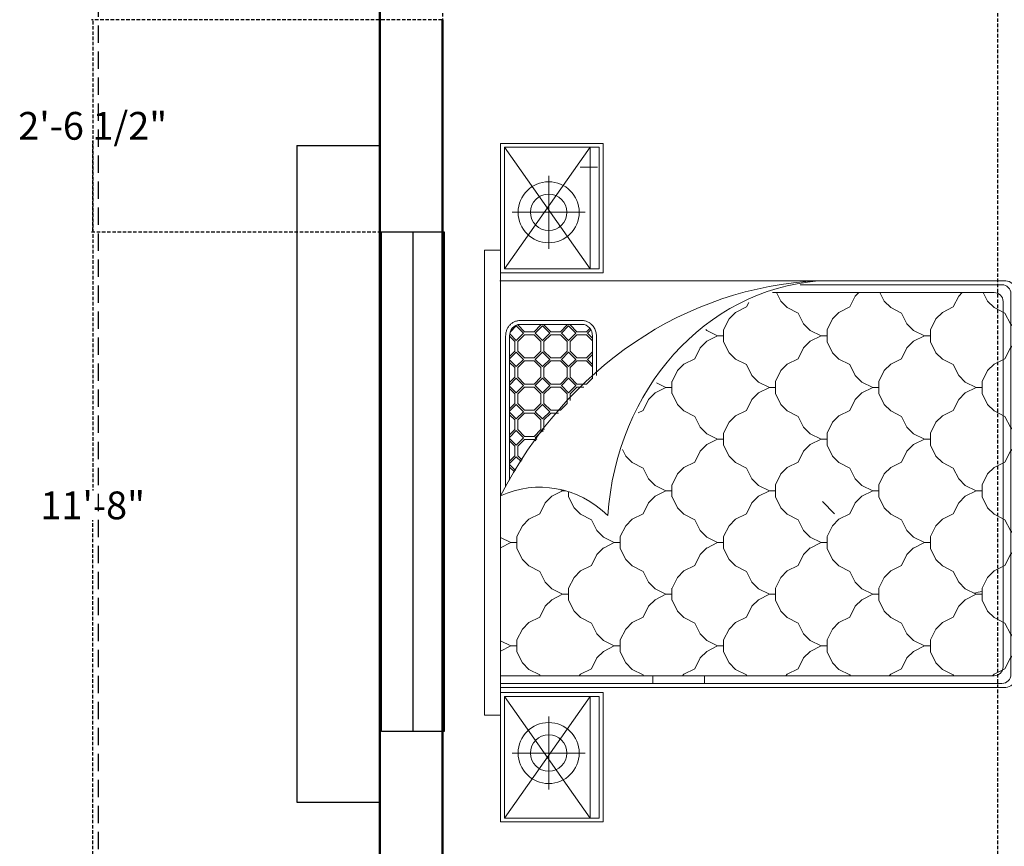
# Model space of a CAD drawing. Units: inches. Extents: x 513 to 1142, y 396 to 927.
# Tile 2 of 31: x 523 to 665, y 518 to 637. Entities that reach past the tile are written whole.
import ezdxf

# ---------------------------------------------------------------- set-up
doc = ezdxf.new("R2010")
doc.units = ezdxf.units.IN
doc.header["$MEASUREMENT"] = 0
doc.linetypes.add('DASHED', pattern=[0.75, 0.5, -0.25])
for name, color, linetype, lineweight in [('A-ANNO-DIMS', 2, 'DASHED', 18), ('A-WALL', 7, 'Continuous', 50), ('furniture', 92, 'Continuous', 18), ('windows', 172, 'Continuous', 25)]:
    doc.layers.add(name, color=color, linetype=linetype, lineweight=lineweight)
doc.styles.get("Standard").update_dxf_attribs({"font": 'arial.ttf'})
doc.dimstyles.get("Standard").update_dxf_attribs({"dimtxt": 4, "dimasz": 0.18, "dimexe": 0.18, "dimexo": 0.0625, "dimgap": 0.09, "dimtad": 0, "dimtih": 1, "dimtoh": 1, "dimdec": 0, "dimrnd": 6, "dimzin": 0, "dimdsep": 46, "dimlunit": 3, "dimtxsty": 'Standard', "dimcen": 0.09, "dimadec": 0, "dimazin": 0, "dimtfac": 1, "dimtdec": 0, "dimtofl": 0, "dimtmove": 0, "dimatfit": 3, "dimfxl": 1, "dimtolj": 1, "dimtzin": 0, "dimarcsym": 0})

# ---------------------------------------------------------------- blocks, each defined once
blk = doc.blocks.new('A$C029D5C69')
for p, q in [((0.4164, 2.0693), (0.4164, 2.0066)), ((2.2315, 2.0693), (0.4164, 2.0693)), ((2.2315, 2.0066), (2.2315, 2.0693)), ((0, 1.606), (0, 2.0066)), ((0, 2.0066), (0.505, 2.0066)), ((0.4164, 2.0066), (2.2315, 2.0066)), ((0.505, 2.0066), (0.505, 1.606)), ((0.5252, 0.0351), (0.5252, 2.0066)), ((0.5403, 0.0502), (0.5403, 2.0066)), ((0.5706, 0.0805), (0.5706, 2.0066)), ((0.6869, 1.966), (0.6666, 2.0066)), ((0.7072, 2.0066), (0.6869, 1.966)), ((1.0902, 1.966), (1.0699, 2.0066)), ((1.1106, 2.0066), (1.0902, 1.966)), ((2.1114, 2.0087), (2.1114, 0.0351)), ((2.6479, 2.0066), (2.1429, 2.0066)), ((2.1429, 2.0066), (2.1429, 1.606)), ((2.6479, 1.606), (2.6479, 2.0066)), ((0.0151, 1.6211), (0.0151, 1.9915)), ((0.0151, 1.9915), (0.4899, 1.9915)), ((0.2689, 1.9609), (0.2689, 1.6764)), ((0.4899, 1.9915), (0.4899, 1.6211)), ((0.6869, 1.9425), (0.6869, 1.966)), ((0.6869, 1.9425), (0.6869, 1.966)), ((1.0902, 1.9425), (1.0902, 1.966)), ((1.0902, 1.9425), (1.0902, 1.966)), ((1.8954, 1.9865), (1.3081, 1.9865)), ((1.8954, 1.9713), (1.3339, 1.9713)), ((1.3849, 1.9713), (1.3656, 1.952)), ((1.3945, 1.9713), (1.3714, 1.9483)), ((1.4249, 1.945), (1.3986, 1.9713)), ((1.4288, 1.9507), (1.4081, 1.9713)), ((1.487, 1.9713), (1.4664, 1.9507)), ((1.4966, 1.9713), (1.4703, 1.945)), ((1.527, 1.945), (1.5007, 1.9713)), ((1.5309, 1.9507), (1.5102, 1.9713)), ((1.5891, 1.9713), (1.5685, 1.9507)), ((1.5987, 1.9713), (1.5724, 1.945)), ((1.6291, 1.945), (1.6028, 1.9713)), ((1.633, 1.9507), (1.6123, 1.9713)), ((1.6912, 1.9713), (1.6706, 1.9507)), ((1.7008, 1.9713), (1.6745, 1.945)), ((1.7312, 1.945), (1.7049, 1.9713)), ((1.7351, 1.9507), (1.7144, 1.9713)), ((1.7933, 1.9713), (1.7727, 1.9507)), ((1.8029, 1.9713), (1.7766, 1.945)), ((1.8333, 1.945), (1.807, 1.9713)), ((1.8372, 1.9507), (1.8165, 1.9713)), ((1.8954, 1.9713), (1.8748, 1.9507)), ((1.9043, 1.9707), (1.8787, 1.945)), ((1.9354, 1.945), (1.9114, 1.969)), ((2.6328, 1.9915), (2.158, 1.9915)), ((2.158, 1.9915), (2.158, 1.6211)), ((2.379, 1.9609), (2.379, 1.6764)), ((2.6328, 1.6211), (2.6328, 1.9915)), ((0.621, 1.9213), (0.5955, 1.8958)), ((0.6634, 1.9425), (0.621, 1.9213)), ((0.6634, 1.9425), (0.621, 1.9213)), ((0.6869, 1.9425), (0.6634, 1.9425)), ((0.6869, 1.9425), (0.7104, 1.9425)), ((0.7528, 1.9213), (0.7104, 1.9425)), ((0.7528, 1.9213), (0.7104, 1.9425)), ((0.7783, 1.8958), (0.7528, 1.9213)), ((1.0243, 1.9213), (0.9988, 1.8958)), ((1.0668, 1.9425), (1.0244, 1.9213)), ((1.0668, 1.9425), (1.0244, 1.9213)), ((1.0902, 1.9425), (1.0668, 1.9425)), ((1.0902, 1.9425), (1.1137, 1.9425)), ((1.1561, 1.9213), (1.1137, 1.9425)), ((1.1561, 1.9213), (1.1137, 1.9425)), ((1.1816, 1.8958), (1.1561, 1.9213)), ((1.4249, 1.945), (1.4059, 1.926)), ((1.4288, 1.9394), (1.4116, 1.9222)), ((1.4476, 1.9507), (1.4288, 1.9507)), ((1.4288, 1.9393), (1.4476, 1.9393)), ((1.4476, 1.9507), (1.4664, 1.9507)), ((1.4664, 1.9393), (1.4476, 1.9393)), ((1.493, 1.9128), (1.4664, 1.9394)), ((1.4986, 1.9167), (1.4703, 1.945)), ((1.527, 1.945), (1.4986, 1.9167)), ((1.5309, 1.9394), (1.5043, 1.9128)), ((1.5497, 1.9507), (1.5309, 1.9507)), ((1.5309, 1.9393), (1.5497, 1.9393)), ((1.5497, 1.9507), (1.5685, 1.9507)), ((1.5685, 1.9393), (1.5497, 1.9393)), ((1.595, 1.9128), (1.5685, 1.9394)), ((1.6007, 1.9167), (1.5724, 1.945)), ((1.6291, 1.945), (1.6007, 1.9167)), ((1.633, 1.9394), (1.6064, 1.9128)), ((1.6518, 1.9507), (1.633, 1.9507)), ((1.633, 1.9393), (1.6518, 1.9393)), ((1.6518, 1.9507), (1.6706, 1.9507)), ((1.6706, 1.9393), (1.6518, 1.9393)), ((1.6971, 1.9128), (1.6706, 1.9394)), ((1.7028, 1.9167), (1.6745, 1.945)), ((1.7312, 1.945), (1.7028, 1.9167)), ((1.7351, 1.9394), (1.7085, 1.9128)), ((1.7539, 1.9507), (1.7351, 1.9507)), ((1.7351, 1.9393), (1.7539, 1.9393)), ((1.7539, 1.9507), (1.7727, 1.9507)), ((1.7727, 1.9393), (1.7539, 1.9393)), ((1.7992, 1.9128), (1.7727, 1.9394)), ((1.8049, 1.9167), (1.7766, 1.945)), ((1.8333, 1.945), (1.8049, 1.9167)), ((1.8372, 1.9394), (1.8106, 1.9128)), ((1.856, 1.9507), (1.8372, 1.9507)), ((1.8372, 1.9393), (1.856, 1.9393)), ((1.856, 1.9507), (1.8748, 1.9507)), ((1.8748, 1.9393), (1.856, 1.9393)), ((1.9013, 1.9128), (1.8748, 1.9394)), ((1.907, 1.9167), (1.8787, 1.945)), ((1.9354, 1.945), (1.907, 1.9167)), ((1.9393, 1.9394), (1.9127, 1.9128)), ((1.9393, 1.9393), (1.9404, 1.9393)), ((1.9414, 1.688), (1.9414, 1.931)), ((1.9565, 1.688), (1.9565, 1.931)), ((0.5955, 1.8958), (0.5743, 1.8534)), ((0.7995, 1.8534), (0.7783, 1.8958)), ((0.9989, 1.8958), (0.9777, 1.8534)), ((1.2028, 1.8534), (1.1816, 1.8958)), ((1.493, 1.8752), (1.493, 1.9128)), ((1.5043, 1.8752), (1.5043, 1.9128)), ((1.595, 1.8752), (1.595, 1.9128)), ((1.6064, 1.8752), (1.6064, 1.9128)), ((1.6971, 1.8752), (1.6971, 1.9128)), ((1.7085, 1.8752), (1.7085, 1.9128)), ((1.7992, 1.8752), (1.7992, 1.9128)), ((1.8106, 1.8752), (1.8106, 1.9128)), ((1.9013, 1.8752), (1.9013, 1.9128)), ((1.9127, 1.8752), (1.9127, 1.9128)), ((0.5743, 1.8534), (0.5706, 1.8515)), ((0.5743, 1.8534), (0.5706, 1.8515)), ((0.8419, 1.8322), (0.7995, 1.8534)), ((0.8419, 1.8322), (0.7995, 1.8534)), ((0.9777, 1.8534), (0.9353, 1.8322)), ((0.9777, 1.8534), (0.9353, 1.8322)), ((1.2452, 1.8322), (1.2028, 1.8534)), ((1.2452, 1.8322), (1.2028, 1.8534)), ((1.493, 1.8752), (1.4867, 1.869)), ((1.4986, 1.8713), (1.4922, 1.8648)), ((1.527, 1.8429), (1.4986, 1.8713)), ((1.5309, 1.8486), (1.5043, 1.8752)), ((1.5497, 1.8486), (1.5309, 1.8486)), ((1.5497, 1.8486), (1.5685, 1.8486)), ((1.595, 1.8752), (1.5685, 1.8486)), ((1.6007, 1.8713), (1.5724, 1.8429)), ((1.6291, 1.8429), (1.6007, 1.8713)), ((1.633, 1.8486), (1.6064, 1.8752)), ((1.6518, 1.8486), (1.633, 1.8486)), ((1.6518, 1.8486), (1.6706, 1.8486)), ((1.6971, 1.8752), (1.6706, 1.8486)), ((1.7028, 1.8713), (1.6745, 1.8429)), ((1.7312, 1.8429), (1.7028, 1.8713)), ((1.7351, 1.8486), (1.7085, 1.8752)), ((1.7539, 1.8486), (1.7351, 1.8486)), ((1.7539, 1.8486), (1.7727, 1.8486)), ((1.7992, 1.8752), (1.7727, 1.8486)), ((1.8049, 1.8713), (1.7766, 1.8429)), ((1.8333, 1.8429), (1.8049, 1.8713)), ((1.8372, 1.8486), (1.8106, 1.8752)), ((1.856, 1.8486), (1.8372, 1.8486)), ((1.856, 1.8486), (1.8748, 1.8486)), ((1.9013, 1.8752), (1.8748, 1.8486)), ((1.907, 1.8713), (1.8787, 1.8429)), ((1.9354, 1.8429), (1.907, 1.8713)), ((1.9393, 1.8486), (1.9127, 1.8752)), ((1.9414, 1.8486), (1.9393, 1.8486)), ((0.1267, 1.8186), (0.4111, 1.8186)), ((0.8674, 1.8067), (0.8419, 1.8322)), ((0.8886, 1.7643), (0.8674, 1.8067)), ((0.9098, 1.8067), (0.8886, 1.7643)), ((0.9352, 1.8322), (0.9097, 1.8067)), ((1.2707, 1.8067), (1.2452, 1.8322)), ((1.2919, 1.7643), (1.2707, 1.8067)), ((1.527, 1.8429), (1.5242, 1.8401)), ((1.5309, 1.8373), (1.5295, 1.8359)), ((1.5309, 1.8373), (1.5497, 1.8373)), ((1.5685, 1.8373), (1.5497, 1.8373)), ((1.595, 1.8107), (1.5685, 1.8373)), ((1.6007, 1.8146), (1.5724, 1.8429)), ((1.595, 1.7806), (1.595, 1.8107)), ((1.6291, 1.8429), (1.6007, 1.8146)), ((1.633, 1.8373), (1.6064, 1.8107)), ((1.6064, 1.7731), (1.6064, 1.8107)), ((1.633, 1.8373), (1.6518, 1.8373)), ((1.6706, 1.8373), (1.6518, 1.8373)), ((1.6971, 1.8107), (1.6706, 1.8373)), ((1.7028, 1.8146), (1.6745, 1.8429)), ((1.6971, 1.7731), (1.6971, 1.8107)), ((1.7312, 1.8429), (1.7028, 1.8146)), ((1.7351, 1.8373), (1.7085, 1.8107)), ((1.7085, 1.7731), (1.7085, 1.8107)), ((1.7351, 1.8373), (1.7539, 1.8373)), ((1.7727, 1.8373), (1.7539, 1.8373)), ((1.7992, 1.8107), (1.7727, 1.8373)), ((1.8049, 1.8146), (1.7766, 1.8429)), ((1.7992, 1.7731), (1.7992, 1.8107)), ((1.8333, 1.8429), (1.8049, 1.8146)), ((1.8372, 1.8373), (1.8106, 1.8107)), ((1.8106, 1.7731), (1.8106, 1.8107)), ((1.8372, 1.8373), (1.856, 1.8373)), ((1.8748, 1.8373), (1.856, 1.8373)), ((1.9013, 1.8107), (1.8748, 1.8373)), ((1.907, 1.8146), (1.8787, 1.8429)), ((1.9013, 1.7731), (1.9013, 1.8107)), ((1.9354, 1.8429), (1.907, 1.8146)), ((1.9393, 1.8373), (1.9127, 1.8107)), ((1.9127, 1.7731), (1.9127, 1.8107)), ((1.9393, 1.8373), (1.9414, 1.8373)), ((2.2367, 1.8186), (2.5212, 1.8186)), ((1.2981, 1.7768), (1.2919, 1.7643)), ((1.633, 1.7465), (1.6064, 1.7731)), ((1.6971, 1.7731), (1.6706, 1.7465)), ((1.7028, 1.7692), (1.6745, 1.7408)), ((1.7312, 1.7408), (1.7028, 1.7692)), ((1.7351, 1.7465), (1.7085, 1.7731)), ((1.7992, 1.7731), (1.7727, 1.7465)), ((1.8049, 1.7692), (1.7766, 1.7408)), ((1.8333, 1.7408), (1.8049, 1.7692)), ((1.8372, 1.7465), (1.8106, 1.7731)), ((1.9013, 1.7731), (1.8748, 1.7465)), ((1.907, 1.7692), (1.8787, 1.7408)), ((1.9354, 1.7408), (1.907, 1.7692)), ((1.9393, 1.7465), (1.9127, 1.7731)), ((0.8651, 1.7408), (0.8227, 1.7196)), ((0.8651, 1.7408), (0.8227, 1.7196)), ((0.912, 1.7408), (0.8651, 1.7408)), ((0.8886, 1.7408), (0.8886, 1.7643)), ((0.9544, 1.7196), (0.912, 1.7408)), ((0.9544, 1.7196), (0.912, 1.7408)), ((1.2684, 1.7408), (1.226, 1.7196)), ((1.2684, 1.7408), (1.226, 1.7196)), ((1.2885, 1.7408), (1.2684, 1.7408)), ((1.2919, 1.7519), (1.2919, 1.7643)), ((1.6518, 1.7465), (1.633, 1.7465)), ((1.6443, 1.7352), (1.6518, 1.7352)), ((1.6518, 1.7465), (1.6706, 1.7465)), ((1.6706, 1.7352), (1.6518, 1.7352)), ((1.6971, 1.7086), (1.6706, 1.7352)), ((1.7028, 1.7125), (1.6745, 1.7408)), ((1.7312, 1.7408), (1.7028, 1.7125)), ((1.7351, 1.7352), (1.7085, 1.7086)), ((1.7539, 1.7465), (1.7351, 1.7465)), ((1.7351, 1.7352), (1.7539, 1.7352)), ((1.7539, 1.7465), (1.7727, 1.7465)), ((1.7727, 1.7352), (1.7539, 1.7352)), ((1.7992, 1.7086), (1.7727, 1.7352)), ((1.8049, 1.7125), (1.7766, 1.7408)), ((1.8333, 1.7408), (1.8049, 1.7125)), ((1.8372, 1.7352), (1.8106, 1.7086)), ((1.856, 1.7465), (1.8372, 1.7465)), ((1.8372, 1.7352), (1.856, 1.7352)), ((1.856, 1.7465), (1.8748, 1.7465)), ((1.8748, 1.7352), (1.856, 1.7352)), ((1.9013, 1.7086), (1.8748, 1.7352)), ((1.907, 1.7125), (1.8787, 1.7408)), ((1.9354, 1.7408), (1.907, 1.7125)), ((1.9393, 1.7352), (1.9127, 1.7086)), ((1.9414, 1.7465), (1.9393, 1.7465)), ((1.9393, 1.7352), (1.9414, 1.7352)), ((0.5766, 1.6941), (0.5706, 1.7002)), ((0.5978, 1.6517), (0.5766, 1.6941)), ((0.7972, 1.6941), (0.776, 1.6517)), ((0.8227, 1.7196), (0.7972, 1.6941)), ((0.98, 1.6941), (0.9545, 1.7196)), ((1.0011, 1.6517), (0.9799, 1.6941)), ((1.2005, 1.6941), (1.1793, 1.6517)), ((1.226, 1.7196), (1.2005, 1.6941)), ((1.6971, 1.682), (1.6971, 1.7086)), ((1.7085, 1.671), (1.7085, 1.7086)), ((1.7992, 1.671), (1.7992, 1.7086)), ((1.8106, 1.671), (1.8106, 1.7086)), ((1.9013, 1.671), (1.9013, 1.7086)), ((1.9127, 1.671), (1.9127, 1.7086)), ((2.5551, 1.6275), (2.5551, 1.696)), ((1.7318, 1.6477), (1.7085, 1.671)), ((1.7992, 1.671), (1.7759, 1.6477)), ((1.8049, 1.6671), (1.7855, 1.6477)), ((1.8244, 1.6477), (1.8049, 1.6671)), ((1.8339, 1.6477), (1.8106, 1.671)), ((1.9013, 1.671), (1.878, 1.6477)), ((1.907, 1.6671), (1.8876, 1.6477)), ((1.9202, 1.6539), (1.907, 1.6671)), ((1.926, 1.6577), (1.9127, 1.671)), ((0.4899, 1.6211), (0.0151, 1.6211)), ((0.6402, 1.6305), (0.5978, 1.6517)), ((0.6402, 1.6305), (0.5978, 1.6517)), ((0.6657, 1.605), (0.6402, 1.6305)), ((0.7336, 1.6305), (0.7081, 1.605)), ((0.776, 1.6517), (0.7336, 1.6305)), ((0.776, 1.6517), (0.7336, 1.6305)), ((1.0435, 1.6305), (1.0011, 1.6517)), ((1.0435, 1.6305), (1.0011, 1.6517)), ((1.0691, 1.605), (1.0436, 1.6305)), ((1.1369, 1.6305), (1.1114, 1.605)), ((1.1793, 1.6517), (1.1369, 1.6305)), ((1.1793, 1.6517), (1.1369, 1.6305)), ((1.8961, 1.6477), (1.7289, 1.6477)), ((1.8961, 1.6325), (1.7422, 1.6325)), ((2.158, 1.6211), (2.6328, 1.6211)), ((0.505, 1.606), (0, 1.606)), ((0.6869, 1.5626), (0.6657, 1.605)), ((0.7081, 1.605), (0.6869, 1.5626)), ((1.0902, 1.5626), (1.069, 1.605)), ((1.1114, 1.605), (1.0902, 1.5626)), ((2.1429, 1.606), (2.6479, 1.606)), ((0.6634, 1.5391), (0.621, 1.5179)), ((0.6634, 1.5391), (0.621, 1.5179)), ((0.6869, 1.5392), (0.6634, 1.5392)), ((0.6869, 1.5392), (0.6869, 1.5626)), ((0.6869, 1.5392), (0.6869, 1.5626)), ((0.6869, 1.5392), (0.7104, 1.5392)), ((0.7528, 1.5179), (0.7104, 1.5391)), ((0.7528, 1.5179), (0.7104, 1.5391)), ((1.0668, 1.5391), (1.0244, 1.5179)), ((1.0668, 1.5391), (1.0244, 1.5179)), ((1.0902, 1.5392), (1.0668, 1.5392)), ((1.0902, 1.5392), (1.0902, 1.5626)), ((1.0902, 1.5392), (1.0902, 1.5626)), ((1.0902, 1.5392), (1.1137, 1.5392)), ((1.1561, 1.5179), (1.1137, 1.5391)), ((1.1561, 1.5179), (1.1137, 1.5391)), ((0.621, 1.5179), (0.5955, 1.4924)), ((0.7783, 1.4924), (0.7528, 1.5179)), ((1.0243, 1.5179), (0.9988, 1.4924)), ((1.1816, 1.4924), (1.1561, 1.5179)), ((1.4277, 1.5179), (1.4022, 1.4924)), ((1.4534, 1.5308), (1.4277, 1.5179)), ((1.4534, 1.5308), (1.4277, 1.5179)), ((0.5955, 1.4925), (0.5743, 1.4501)), ((0.7995, 1.4501), (0.7783, 1.4925)), ((0.9989, 1.4925), (0.9777, 1.4501)), ((1.2028, 1.4501), (1.1816, 1.4925)), ((1.4022, 1.4925), (1.381, 1.4501)), ((1.6062, 1.4501), (1.5966, 1.4692)), ((0.5743, 1.45), (0.5706, 1.4481)), ((0.5743, 1.45), (0.5706, 1.4481)), ((0.8419, 1.4288), (0.7995, 1.45)), ((0.8419, 1.4288), (0.7995, 1.45)), ((0.8674, 1.4033), (0.8419, 1.4288)), ((0.9352, 1.4288), (0.9097, 1.4033)), ((0.9777, 1.45), (0.9353, 1.4288)), ((0.9777, 1.45), (0.9353, 1.4288)), ((1.2452, 1.4288), (1.2028, 1.45)), ((1.2452, 1.4288), (1.2028, 1.45)), ((1.2707, 1.4033), (1.2452, 1.4288)), ((1.3386, 1.4288), (1.3131, 1.4033)), ((1.381, 1.45), (1.3386, 1.4288)), ((1.381, 1.45), (1.3386, 1.4288)), ((1.6486, 1.4288), (1.6062, 1.45)), ((1.6486, 1.4288), (1.6062, 1.45)), ((1.6741, 1.4033), (1.6486, 1.4288)), ((0.5403, 1.4117), (0.5706, 1.4117)), ((0.8886, 1.361), (0.8674, 1.4034)), ((0.9098, 1.4034), (0.8886, 1.361)), ((1.2919, 1.361), (1.2707, 1.4034)), ((1.3131, 1.4034), (1.2919, 1.361)), ((1.6953, 1.361), (1.6741, 1.4034)), ((1.714, 1.3984), (1.6953, 1.361)), ((0.8886, 1.3375), (0.8886, 1.3609)), ((1.2919, 1.3375), (1.2919, 1.3609)), ((1.6953, 1.3375), (1.6953, 1.3609)), ((0.8227, 1.3163), (0.7972, 1.2908)), ((0.8651, 1.3374), (0.8227, 1.3162)), ((0.8651, 1.3374), (0.8227, 1.3162)), ((0.912, 1.3375), (0.8651, 1.3375)), ((0.9544, 1.3162), (0.912, 1.3374)), ((0.9544, 1.3162), (0.912, 1.3374)), ((0.98, 1.2908), (0.9545, 1.3163)), ((1.226, 1.3163), (1.2005, 1.2908)), ((1.2684, 1.3374), (1.226, 1.3162)), ((1.2684, 1.3374), (1.226, 1.3162)), ((1.3154, 1.3375), (1.2684, 1.3375)), ((1.3578, 1.3162), (1.3154, 1.3374)), ((1.3578, 1.3162), (1.3154, 1.3374)), ((1.3833, 1.2908), (1.3578, 1.3163)), ((1.6294, 1.3163), (1.6039, 1.2908)), ((1.6718, 1.3374), (1.6294, 1.3162)), ((1.6718, 1.3374), (1.6294, 1.3162)), ((1.7187, 1.3375), (1.6718, 1.3375)), ((1.7611, 1.3162), (1.7187, 1.3374)), ((1.7611, 1.3162), (1.7187, 1.3374)), ((1.7867, 1.2908), (1.7611, 1.3163)), ((0.5766, 1.2908), (0.5706, 1.2968)), ((0.5978, 1.2484), (0.5766, 1.2908)), ((0.7972, 1.2908), (0.776, 1.2484)), ((1.0011, 1.2484), (0.9799, 1.2908)), ((1.2005, 1.2908), (1.1793, 1.2484)), ((1.4045, 1.2484), (1.3833, 1.2908)), ((1.6039, 1.2908), (1.5827, 1.2484)), ((1.8078, 1.2484), (1.7866, 1.2908)), ((0.6402, 1.2271), (0.5978, 1.2483)), ((0.6402, 1.2271), (0.5978, 1.2483)), ((0.776, 1.2483), (0.7336, 1.2271)), ((0.776, 1.2483), (0.7336, 1.2271)), ((1.0435, 1.2271), (1.0011, 1.2483)), ((1.0435, 1.2271), (1.0011, 1.2483)), ((1.1793, 1.2483), (1.1369, 1.2271)), ((1.1793, 1.2483), (1.1369, 1.2271)), ((1.4469, 1.2271), (1.4045, 1.2483)), ((1.4469, 1.2271), (1.4045, 1.2483)), ((1.5827, 1.2483), (1.5403, 1.2271)), ((1.5827, 1.2483), (1.5403, 1.2271)), ((1.8502, 1.2271), (1.8078, 1.2483)), ((1.8502, 1.2271), (1.8078, 1.2483)), ((0.5403, 1.21), (0.5706, 1.21)), ((0.6657, 1.2017), (0.6402, 1.2272)), ((0.6869, 1.1593), (0.6657, 1.2017)), ((0.7081, 1.2017), (0.6869, 1.1593)), ((0.7336, 1.2272), (0.7081, 1.2017)), ((1.0691, 1.2017), (1.0436, 1.2272)), ((1.0902, 1.1593), (1.069, 1.2017)), ((1.1114, 1.2017), (1.0902, 1.1593)), ((1.1369, 1.2272), (1.1114, 1.2017)), ((1.4724, 1.2017), (1.4469, 1.2272)), ((1.4936, 1.1593), (1.4724, 1.2017)), ((1.5148, 1.2017), (1.4936, 1.1593)), ((1.5403, 1.2272), (1.5148, 1.2017)), ((1.8758, 1.2017), (1.8503, 1.2272)), ((1.8969, 1.1593), (1.8757, 1.2017)), ((1.9181, 1.2017), (1.8969, 1.1593)), ((1.9215, 1.2051), (1.9181, 1.2017)), ((0.6869, 1.1358), (0.6869, 1.1593)), ((0.6869, 1.1358), (0.6869, 1.1593)), ((1.0902, 1.1358), (1.0902, 1.1593)), ((1.0902, 1.1358), (1.0902, 1.1593)), ((1.4936, 1.1358), (1.4936, 1.1593)), ((1.4936, 1.1358), (1.4936, 1.1593)), ((1.8969, 1.1358), (1.8969, 1.1593)), ((1.8969, 1.1358), (1.8969, 1.1593)), ((0.621, 1.1146), (0.5955, 1.0891)), ((0.6634, 1.1358), (0.621, 1.1146)), ((0.6634, 1.1358), (0.621, 1.1146)), ((0.6869, 1.1358), (0.6634, 1.1358)), ((0.6869, 1.1358), (0.7104, 1.1358)), ((0.7528, 1.1146), (0.7104, 1.1358)), ((0.7528, 1.1146), (0.7104, 1.1358)), ((0.7783, 1.0891), (0.7528, 1.1146)), ((1.0243, 1.1146), (0.9988, 1.0891)), ((1.0668, 1.1358), (1.0244, 1.1146)), ((1.0668, 1.1358), (1.0244, 1.1146)), ((1.0902, 1.1358), (1.0668, 1.1358)), ((1.0902, 1.1358), (1.1137, 1.1358)), ((1.1561, 1.1146), (1.1137, 1.1358)), ((1.1561, 1.1146), (1.1137, 1.1358)), ((1.1816, 1.0891), (1.1561, 1.1146)), ((1.4277, 1.1146), (1.4022, 1.0891)), ((1.4701, 1.1358), (1.4277, 1.1146)), ((1.4701, 1.1358), (1.4277, 1.1146)), ((1.4936, 1.1358), (1.4701, 1.1358)), ((1.4936, 1.1358), (1.5171, 1.1358)), ((1.5595, 1.1146), (1.5171, 1.1358)), ((1.5595, 1.1146), (1.5171, 1.1358)), ((1.585, 1.0891), (1.5595, 1.1146)), ((1.831, 1.1146), (1.8055, 1.0891)), ((1.8735, 1.1358), (1.8311, 1.1146)), ((1.8735, 1.1358), (1.8311, 1.1146)), ((1.8969, 1.1358), (1.8735, 1.1358)), ((1.8969, 1.1358), (1.9204, 1.1358)), ((1.9628, 1.1146), (1.9204, 1.1358)), ((1.9628, 1.1146), (1.9204, 1.1358)), ((1.9883, 1.0891), (1.9628, 1.1146)), ((0.5955, 1.0891), (0.5743, 1.0467)), ((0.7995, 1.0467), (0.7783, 1.0891)), ((0.9989, 1.0891), (0.9777, 1.0467)), ((1.2028, 1.0467), (1.1816, 1.0891)), ((1.4022, 1.0891), (1.381, 1.0467)), ((1.6062, 1.0467), (1.585, 1.0891)), ((1.8056, 1.0891), (1.7844, 1.0467)), ((2.0095, 1.0467), (1.9883, 1.0891)), ((0.5743, 1.0467), (0.5706, 1.0448)), ((0.5743, 1.0467), (0.5706, 1.0448)), ((0.8419, 1.0255), (0.7995, 1.0467)), ((0.8419, 1.0255), (0.7995, 1.0467)), ((0.9777, 1.0467), (0.9353, 1.0255)), ((0.9777, 1.0467), (0.9353, 1.0255)), ((1.2452, 1.0255), (1.2028, 1.0467)), ((1.2452, 1.0255), (1.2028, 1.0467)), ((1.381, 1.0467), (1.3386, 1.0255)), ((1.381, 1.0467), (1.3386, 1.0255)), ((1.6486, 1.0255), (1.6062, 1.0467)), ((1.6486, 1.0255), (1.6062, 1.0467)), ((1.7844, 1.0467), (1.742, 1.0255)), ((1.7844, 1.0467), (1.742, 1.0255)), ((2.0276, 1.0376), (2.0095, 1.0467)), ((2.0276, 1.0376), (2.0095, 1.0467)), ((0.8674, 1), (0.8419, 1.0255)), ((0.8886, 0.9576), (0.8674, 1)), ((0.9098, 1), (0.8886, 0.9576)), ((0.9352, 1.0255), (0.9097, 1)), ((1.2707, 1), (1.2452, 1.0255)), ((1.2919, 0.9576), (1.2707, 1)), ((1.3131, 1), (1.2919, 0.9576)), ((1.3386, 1.0255), (1.3131, 1)), ((1.6741, 1), (1.6486, 1.0255)), ((1.6953, 0.9576), (1.6741, 1)), ((1.7165, 1), (1.6953, 0.9576)), ((1.7419, 1.0255), (1.7164, 1)), ((0.8651, 0.9341), (0.8227, 0.9129)), ((0.8651, 0.9341), (0.8227, 0.9129)), ((0.912, 0.9341), (0.8651, 0.9341)), ((0.8886, 0.9341), (0.8886, 0.9576)), ((0.9544, 0.9129), (0.912, 0.9341)), ((0.9544, 0.9129), (0.912, 0.9341)), ((1.2684, 0.9341), (1.226, 0.9129)), ((1.2684, 0.9341), (1.226, 0.9129)), ((1.3154, 0.9341), (1.2684, 0.9341)), ((1.2919, 0.9341), (1.2919, 0.9576)), ((1.3578, 0.9129), (1.3154, 0.9341)), ((1.3578, 0.9129), (1.3154, 0.9341)), ((1.6718, 0.9341), (1.6294, 0.9129)), ((1.6718, 0.9341), (1.6294, 0.9129)), ((1.7187, 0.9341), (1.6718, 0.9341)), ((1.6953, 0.9341), (1.6953, 0.9576)), ((1.7611, 0.9129), (1.7187, 0.9341)), ((1.7611, 0.9129), (1.7187, 0.9341)), ((2.066, 0.9295), (2.0327, 0.9129)), ((2.066, 0.9295), (2.0327, 0.9129)), ((2.066, 0.9457), (2.066, 0.0805)), ((0.5766, 0.8874), (0.5706, 0.8935)), ((0.5978, 0.845), (0.5766, 0.8874)), ((0.7972, 0.8874), (0.776, 0.845)), ((0.8227, 0.9129), (0.7972, 0.8874)), ((0.98, 0.8874), (0.9545, 0.9129)), ((1.0011, 0.845), (0.9799, 0.8874)), ((1.2005, 0.8874), (1.1793, 0.845)), ((1.226, 0.9129), (1.2005, 0.8874)), ((1.3833, 0.8874), (1.3578, 0.9129)), ((1.4045, 0.845), (1.3833, 0.8874)), ((1.6039, 0.8874), (1.5827, 0.845)), ((1.6294, 0.9129), (1.6039, 0.8874)), ((1.7867, 0.8874), (1.7611, 0.9129)), ((1.8078, 0.845), (1.7866, 0.8874)), ((2.0072, 0.8874), (1.986, 0.845)), ((2.0327, 0.9129), (2.0072, 0.8874)), ((0.6402, 0.8238), (0.5978, 0.845)), ((0.6402, 0.8238), (0.5978, 0.845)), ((0.6657, 0.7983), (0.6402, 0.8238)), ((0.7336, 0.8238), (0.7081, 0.7983)), ((0.776, 0.845), (0.7336, 0.8238)), ((0.776, 0.845), (0.7336, 0.8238)), ((1.0435, 0.8238), (1.0011, 0.845)), ((1.0435, 0.8238), (1.0011, 0.845)), ((1.0691, 0.7983), (1.0436, 0.8238)), ((1.1369, 0.8238), (1.1114, 0.7983)), ((1.1793, 0.845), (1.1369, 0.8238)), ((1.1793, 0.845), (1.1369, 0.8238)), ((1.4469, 0.8238), (1.4045, 0.845)), ((1.4469, 0.8238), (1.4045, 0.845)), ((1.4724, 0.7983), (1.4469, 0.8238)), ((1.5403, 0.8238), (1.5148, 0.7983)), ((1.5827, 0.845), (1.5403, 0.8238)), ((1.5827, 0.845), (1.5403, 0.8238)), ((1.8502, 0.8238), (1.8078, 0.845)), ((1.8502, 0.8238), (1.8078, 0.845)), ((1.8758, 0.7983), (1.8503, 0.8238)), ((1.9436, 0.8238), (1.9181, 0.7983)), ((1.986, 0.845), (1.9436, 0.8238)), ((1.986, 0.845), (1.9436, 0.8238)), ((2.0962, 0.8369), (2.0962, 0.0502)), ((0.6869, 0.7559), (0.6657, 0.7983)), ((0.7081, 0.7983), (0.6869, 0.7559)), ((1.0902, 0.7559), (1.069, 0.7983)), ((1.1114, 0.7983), (1.0902, 0.7559)), ((1.4936, 0.7559), (1.4724, 0.7983)), ((1.5148, 0.7983), (1.4936, 0.7559)), ((1.8969, 0.7559), (1.8757, 0.7983)), ((1.9181, 0.7983), (1.8969, 0.7559)), ((0.6634, 0.7324), (0.621, 0.7112)), ((0.6634, 0.7324), (0.621, 0.7112)), ((0.6869, 0.7325), (0.6634, 0.7325)), ((0.6869, 0.7325), (0.6869, 0.7559)), ((0.6869, 0.7325), (0.6869, 0.7559)), ((0.6869, 0.7325), (0.7104, 0.7325)), ((0.7528, 0.7112), (0.7104, 0.7324)), ((0.7528, 0.7112), (0.7104, 0.7324)), ((1.0668, 0.7324), (1.0244, 0.7112)), ((1.0668, 0.7324), (1.0244, 0.7112)), ((1.0902, 0.7325), (1.0668, 0.7325)), ((1.0902, 0.7325), (1.0902, 0.7559)), ((1.0902, 0.7325), (1.0902, 0.7559)), ((1.0902, 0.7325), (1.1137, 0.7325)), ((1.1561, 0.7112), (1.1137, 0.7324)), ((1.1561, 0.7112), (1.1137, 0.7324)), ((1.2024, 0.7028), (1.2503, 0.7507)), ((1.4701, 0.7324), (1.4277, 0.7112)), ((1.4701, 0.7324), (1.4277, 0.7112)), ((1.4936, 0.7325), (1.4701, 0.7325)), ((1.4936, 0.7325), (1.4936, 0.7559)), ((1.4936, 0.7325), (1.4936, 0.7559)), ((1.4936, 0.7325), (1.5171, 0.7325)), ((1.5595, 0.7112), (1.5171, 0.7324)), ((1.5595, 0.7112), (1.5171, 0.7324)), ((1.8735, 0.7324), (1.8311, 0.7112)), ((1.8735, 0.7324), (1.8311, 0.7112)), ((1.8969, 0.7325), (1.8735, 0.7325)), ((1.8969, 0.7325), (1.8969, 0.7559)), ((1.8969, 0.7325), (1.8969, 0.7559)), ((1.8969, 0.7325), (1.9204, 0.7325)), ((1.9628, 0.7112), (1.9204, 0.7324)), ((1.9628, 0.7112), (1.9204, 0.7324)), ((0.621, 0.7113), (0.5955, 0.6858)), ((0.7783, 0.6858), (0.7528, 0.7113)), ((1.0243, 0.7113), (0.9988, 0.6858)), ((1.1816, 0.6858), (1.1561, 0.7113)), ((1.4277, 0.7113), (1.4022, 0.6858)), ((1.585, 0.6858), (1.5595, 0.7113)), ((1.831, 0.7113), (1.8055, 0.6858)), ((1.9883, 0.6858), (1.9628, 0.7113)), ((0.5955, 0.6858), (0.5743, 0.6434)), ((0.7995, 0.6434), (0.7783, 0.6858)), ((0.9989, 0.6858), (0.9777, 0.6434)), ((1.2028, 0.6434), (1.1816, 0.6858)), ((1.4022, 0.6858), (1.381, 0.6434)), ((1.6062, 0.6434), (1.585, 0.6858)), ((1.8056, 0.6858), (1.7844, 0.6434)), ((2.0095, 0.6434), (1.9883, 0.6858)), ((0.5743, 0.6433), (0.5706, 0.6414)), ((0.5743, 0.6433), (0.5706, 0.6414)), ((0.8419, 0.6221), (0.7995, 0.6433)), ((0.8419, 0.6221), (0.7995, 0.6433)), ((0.8674, 0.5967), (0.8419, 0.6222)), ((0.9352, 0.6222), (0.9097, 0.5967)), ((0.9777, 0.6433), (0.9353, 0.6221)), ((0.9777, 0.6433), (0.9353, 0.6221)), ((1.2452, 0.6221), (1.2028, 0.6433)), ((1.2452, 0.6221), (1.2028, 0.6433)), ((1.2707, 0.5967), (1.2452, 0.6222)), ((1.3386, 0.6222), (1.3131, 0.5967)), ((1.381, 0.6433), (1.3386, 0.6221)), ((1.381, 0.6433), (1.3386, 0.6221)), ((1.6486, 0.6221), (1.6062, 0.6433)), ((1.6486, 0.6221), (1.6062, 0.6433)), ((1.6741, 0.5967), (1.6486, 0.6222)), ((1.7419, 0.6222), (1.7164, 0.5967)), ((1.7844, 0.6433), (1.742, 0.6221)), ((1.7844, 0.6433), (1.742, 0.6221)), ((2.0519, 0.6221), (2.0095, 0.6433)), ((2.0519, 0.6221), (2.0095, 0.6433)), ((2.066, 0.6081), (2.0519, 0.6222)), ((0.8886, 0.5543), (0.8674, 0.5967)), ((0.9098, 0.5967), (0.8886, 0.5543)), ((1.2919, 0.5543), (1.2707, 0.5967)), ((1.3131, 0.5967), (1.2919, 0.5543)), ((1.6953, 0.5543), (1.6741, 0.5967)), ((1.7165, 0.5967), (1.6953, 0.5543)), ((0.8886, 0.5308), (0.8886, 0.5543)), ((1.2919, 0.5308), (1.2919, 0.5543)), ((1.6953, 0.5308), (1.6953, 0.5543)), ((0.8227, 0.5096), (0.7972, 0.4841)), ((0.8651, 0.5308), (0.8227, 0.5096)), ((0.8651, 0.5308), (0.8227, 0.5096)), ((0.912, 0.5308), (0.8651, 0.5308)), ((0.9544, 0.5096), (0.912, 0.5308)), ((0.9544, 0.5096), (0.912, 0.5308)), ((0.98, 0.4841), (0.9545, 0.5096)), ((1.226, 0.5096), (1.2005, 0.4841)), ((1.2684, 0.5308), (1.226, 0.5096)), ((1.2684, 0.5308), (1.226, 0.5096)), ((1.3154, 0.5308), (1.2684, 0.5308)), ((1.3578, 0.5096), (1.3154, 0.5308)), ((1.3578, 0.5096), (1.3154, 0.5308)), ((1.3833, 0.4841), (1.3578, 0.5096)), ((1.6294, 0.5096), (1.6039, 0.4841)), ((1.6718, 0.5308), (1.6294, 0.5096)), ((1.6718, 0.5308), (1.6294, 0.5096)), ((1.7187, 0.5308), (1.6718, 0.5308)), ((1.7611, 0.5096), (1.7187, 0.5308)), ((1.7611, 0.5096), (1.7187, 0.5308)), ((1.7867, 0.4841), (1.7611, 0.5096)), ((2.0327, 0.5096), (2.0072, 0.4841)), ((2.066, 0.5262), (2.0327, 0.5096)), ((2.066, 0.5262), (2.0327, 0.5096)), ((0.5766, 0.4841), (0.5706, 0.4901)), ((0.5978, 0.4417), (0.5766, 0.4841)), ((0.7972, 0.4841), (0.776, 0.4417)), ((1.0011, 0.4417), (0.9799, 0.4841)), ((1.2005, 0.4841), (1.1793, 0.4417)), ((1.4045, 0.4417), (1.3833, 0.4841)), ((1.6039, 0.4841), (1.5827, 0.4417)), ((1.8078, 0.4417), (1.7866, 0.4841)), ((2.0072, 0.4841), (1.986, 0.4417)), ((0.6402, 0.4205), (0.5978, 0.4417)), ((0.6402, 0.4205), (0.5978, 0.4417)), ((0.776, 0.4417), (0.7336, 0.4205)), ((0.776, 0.4417), (0.7336, 0.4205)), ((1.0435, 0.4205), (1.0011, 0.4417)), ((1.0435, 0.4205), (1.0011, 0.4417)), ((1.1793, 0.4417), (1.1369, 0.4205)), ((1.1793, 0.4417), (1.1369, 0.4205)), ((1.4469, 0.4205), (1.4045, 0.4417)), ((1.4469, 0.4205), (1.4045, 0.4417)), ((1.5827, 0.4417), (1.5403, 0.4205)), ((1.5827, 0.4417), (1.5403, 0.4205)), ((1.8502, 0.4205), (1.8078, 0.4417)), ((1.8502, 0.4205), (1.8078, 0.4417)), ((1.986, 0.4417), (1.9436, 0.4205)), ((1.986, 0.4417), (1.9436, 0.4205)), ((0.6657, 0.395), (0.6402, 0.4205)), ((0.6869, 0.3526), (0.6657, 0.395)), ((0.7081, 0.395), (0.6869, 0.3526)), ((0.7336, 0.4205), (0.7081, 0.395)), ((1.0691, 0.395), (1.0436, 0.4205)), ((1.0902, 0.3526), (1.069, 0.395)), ((1.1114, 0.395), (1.0902, 0.3526)), ((1.1369, 0.4205), (1.1114, 0.395)), ((1.4724, 0.395), (1.4469, 0.4205)), ((1.4936, 0.3526), (1.4724, 0.395)), ((1.5148, 0.395), (1.4936, 0.3526)), ((1.5403, 0.4205), (1.5148, 0.395)), ((1.8758, 0.395), (1.8503, 0.4205)), ((1.8969, 0.3526), (1.8757, 0.395)), ((1.9181, 0.395), (1.8969, 0.3526)), ((1.9436, 0.4205), (1.9181, 0.395)), ((0.6869, 0.3291), (0.6869, 0.3526)), ((0.6869, 0.3291), (0.6869, 0.3526)), ((1.0902, 0.3291), (1.0902, 0.3526)), ((1.0902, 0.3291), (1.0902, 0.3526)), ((1.4936, 0.3291), (1.4936, 0.3526)), ((1.4936, 0.3291), (1.4936, 0.3526)), ((1.8969, 0.3291), (1.8969, 0.3526)), ((1.8969, 0.3291), (1.8969, 0.3526)), ((0.621, 0.3079), (0.5955, 0.2824)), ((0.6634, 0.3291), (0.621, 0.3079)), ((0.6634, 0.3291), (0.621, 0.3079)), ((0.6869, 0.3291), (0.6634, 0.3291)), ((0.6869, 0.3291), (0.7104, 0.3291)), ((0.7528, 0.3079), (0.7104, 0.3291)), ((0.7528, 0.3079), (0.7104, 0.3291)), ((0.7783, 0.2824), (0.7528, 0.3079)), ((1.0243, 0.3079), (0.9988, 0.2824)), ((1.0668, 0.3291), (1.0244, 0.3079)), ((1.0668, 0.3291), (1.0244, 0.3079)), ((1.0902, 0.3291), (1.0668, 0.3291)), ((1.0902, 0.3291), (1.1137, 0.3291)), ((1.1561, 0.3079), (1.1137, 0.3291)), ((1.1561, 0.3079), (1.1137, 0.3291)), ((1.1816, 0.2824), (1.1561, 0.3079)), ((1.4277, 0.3079), (1.4022, 0.2824)), ((1.4701, 0.3291), (1.4277, 0.3079)), ((1.4701, 0.3291), (1.4277, 0.3079)), ((1.4936, 0.3291), (1.4701, 0.3291)), ((1.4936, 0.3291), (1.5171, 0.3291)), ((1.5595, 0.3079), (1.5171, 0.3291)), ((1.5595, 0.3079), (1.5171, 0.3291)), ((1.585, 0.2824), (1.5595, 0.3079)), ((1.831, 0.3079), (1.8055, 0.2824)), ((1.8735, 0.3291), (1.8311, 0.3079)), ((1.8735, 0.3291), (1.8311, 0.3079)), ((1.8969, 0.3291), (1.8735, 0.3291)), ((1.8969, 0.3291), (1.9204, 0.3291)), ((1.9628, 0.3079), (1.9204, 0.3291)), ((1.9628, 0.3079), (1.9204, 0.3291)), ((1.9883, 0.2824), (1.9628, 0.3079)), ((0.5955, 0.2824), (0.5743, 0.24)), ((0.7995, 0.24), (0.7783, 0.2824)), ((0.9989, 0.2824), (0.9777, 0.24)), ((1.2028, 0.24), (1.1816, 0.2824)), ((1.4022, 0.2824), (1.381, 0.24)), ((1.6062, 0.24), (1.585, 0.2824)), ((1.8056, 0.2824), (1.7844, 0.24)), ((2.0095, 0.24), (1.9883, 0.2824)), ((0.5743, 0.24), (0.5706, 0.2381)), ((0.5743, 0.24), (0.5706, 0.2381)), ((0.8419, 0.2188), (0.7995, 0.24)), ((0.8419, 0.2188), (0.7995, 0.24)), ((0.9777, 0.24), (0.9353, 0.2188)), ((0.9777, 0.24), (0.9353, 0.2188)), ((1.2452, 0.2188), (1.2028, 0.24)), ((1.2452, 0.2188), (1.2028, 0.24)), ((1.381, 0.24), (1.3386, 0.2188)), ((1.381, 0.24), (1.3386, 0.2188)), ((1.6486, 0.2188), (1.6062, 0.24)), ((1.6486, 0.2188), (1.6062, 0.24)), ((1.7844, 0.24), (1.742, 0.2188)), ((1.7844, 0.24), (1.742, 0.2188)), ((2.0519, 0.2188), (2.0095, 0.24)), ((2.0519, 0.2188), (2.0095, 0.24)), ((0.8674, 0.1933), (0.8419, 0.2188)), ((0.8886, 0.1509), (0.8674, 0.1933)), ((0.9098, 0.1933), (0.8886, 0.1509)), ((0.9352, 0.2188), (0.9097, 0.1933)), ((1.2707, 0.1933), (1.2452, 0.2188)), ((1.2919, 0.1509), (1.2707, 0.1933)), ((1.3131, 0.1933), (1.2919, 0.1509)), ((1.3386, 0.2188), (1.3131, 0.1933)), ((1.6741, 0.1933), (1.6486, 0.2188)), ((1.6953, 0.1509), (1.6741, 0.1933)), ((1.7165, 0.1933), (1.6953, 0.1509)), ((1.7419, 0.2188), (1.7164, 0.1933)), ((2.066, 0.2047), (2.0519, 0.2188)), ((0.8651, 0.1274), (0.8227, 0.1062)), ((0.8651, 0.1274), (0.8227, 0.1062)), ((0.912, 0.1275), (0.8651, 0.1275)), ((0.8886, 0.1275), (0.8886, 0.1509)), ((0.9544, 0.1062), (0.912, 0.1274)), ((0.9544, 0.1062), (0.912, 0.1274)), ((1.2684, 0.1274), (1.226, 0.1062)), ((1.2684, 0.1274), (1.226, 0.1062)), ((1.3154, 0.1275), (1.2684, 0.1275)), ((1.2919, 0.1275), (1.2919, 0.1509)), ((1.3578, 0.1062), (1.3154, 0.1274)), ((1.3578, 0.1062), (1.3154, 0.1274)), ((1.6718, 0.1274), (1.6294, 0.1062)), ((1.6718, 0.1274), (1.6294, 0.1062)), ((1.7187, 0.1275), (1.6718, 0.1275)), ((1.6953, 0.1275), (1.6953, 0.1509)), ((1.7611, 0.1062), (1.7187, 0.1274)), ((1.7611, 0.1062), (1.7187, 0.1274)), ((2.066, 0.1228), (2.0327, 0.1062)), ((2.066, 0.1228), (2.0327, 0.1062)), ((0.5766, 0.0807), (0.5706, 0.0868)), ((0.5978, 0.0384), (0.5766, 0.0808)), ((0.7972, 0.0808), (0.776, 0.0384)), ((0.8227, 0.1062), (0.7972, 0.0807)), ((0.98, 0.0807), (0.9545, 0.1062)), ((1.0011, 0.0384), (0.9799, 0.0808)), ((1.2005, 0.0808), (1.1793, 0.0384)), ((1.226, 0.1062), (1.2005, 0.0807)), ((1.3833, 0.0807), (1.3578, 0.1062)), ((1.4045, 0.0384), (1.3833, 0.0808)), ((1.6039, 0.0808), (1.5827, 0.0384)), ((1.6294, 0.1062), (1.6039, 0.0807)), ((1.7867, 0.0807), (1.7611, 0.1062)), ((1.8078, 0.0384), (1.7866, 0.0808)), ((2.0072, 0.0808), (1.986, 0.0384)), ((2.0327, 0.1062), (2.0072, 0.0807)), ((2.0309, 0.0454), (0.6056, 0.0454)), ((2.0763, 0), (0.5603, 0)), ((2.0612, 0.0151), (0.5754, 0.0151)), ((0.6402, 0.0171), (0.5978, 0.0383)), ((0.6402, 0.0171), (0.5978, 0.0383)), ((0.6523, 0.005), (0.6402, 0.0171)), ((0.7336, 0.0171), (0.7215, 0.005)), ((0.776, 0.0383), (0.7336, 0.0171)), ((0.776, 0.0383), (0.7336, 0.0171)), ((1.0435, 0.0171), (1.0011, 0.0383)), ((1.0435, 0.0171), (1.0011, 0.0383)), ((1.0557, 0.005), (1.0436, 0.0171)), ((1.1369, 0.0171), (1.1248, 0.005)), ((1.1793, 0.0383), (1.1369, 0.0171)), ((1.1793, 0.0383), (1.1369, 0.0171)), ((1.4469, 0.0171), (1.4045, 0.0383)), ((1.4469, 0.0171), (1.4045, 0.0383)), ((1.459, 0.005), (1.4469, 0.0171)), ((1.5403, 0.0171), (1.5282, 0.005)), ((1.5827, 0.0383), (1.5403, 0.0171)), ((1.5827, 0.0383), (1.5403, 0.0171)), ((1.8502, 0.0171), (1.8078, 0.0383)), ((1.8502, 0.0171), (1.8078, 0.0383)), ((1.8623, 0.005), (1.8503, 0.0171)), ((1.9436, 0.0171), (1.9315, 0.005)), ((1.986, 0.0383), (1.9436, 0.0171)), ((1.986, 0.0383), (1.9436, 0.0171))]:
    blk.add_line(p, q)
at = {"ltscale": 0.005}
for p, q in [((0.4899, 1.6568), (0.0151, 1.9915)), ((0.0151, 1.6568), (0.4899, 1.9915)), ((2.6328, 1.6568), (2.158, 1.9915)), ((2.158, 1.6568), (2.6328, 1.9915)), ((0.0151, 1.6568), (0.4899, 1.6568)), ((2.6328, 1.6568), (2.158, 1.6568))]:
    blk.add_line(p, q, dxfattribs=at)
for centre, radius in [((0.2689, 1.8186), 0.1191), ((2.379, 1.8186), 0.1191), ((0.2689, 1.8186), 0.0711), ((2.379, 1.8186), 0.0711)]:
    blk.add_circle(centre, radius)
for centre, radius, start, end in [((0.2843, 0.0157), 0.6251, 10.2961, 13.2684), ((0.6056, 0.0805), 0.0351, 180, 270), ((2.0309, 0.0805), 0.0351, 270, 0), ((0.5754, 0.0502), 0.0351, 180, 270), ((2.0612, 0.0502), 0.0351, 270, 0), ((0.5603, 0.0351), 0.0351, 180, 270), ((2.0763, 0.0351), 0.0351, 270, 0)]:
    blk.add_arc(centre, radius, start, end)
for centre, major_axis, ratio, start_param, end_param in [((0.8506, 1.8527), (-0.4556, 0), 0.89, 2.430919, 3.53111), ((0.3667, 0.6698), (1.7398, 0.1668), 0.88072, -0.045073, 0.941433), ((1.8961, 1.931), (-0.0453, 0), 0.89, 3.141593, 4.712389), ((1.8961, 1.688), (-0.0453, 0), 0.89, 1.570796, 3.141593), ((1.0874, 0.6748), (1.021, 0.1213), 0.889348, -0.031673, 1.359628)]:
    blk.add_ellipse(centre, major_axis=major_axis, ratio=ratio, start_param=start_param, end_param=end_param)
for points, knots in [([(1.9565, 1.931), (1.9565, 1.9336), (1.9563, 1.9362), (1.9553, 1.9428), (1.9543, 1.9467), (1.9512, 1.9541), (1.9493, 1.9577), (1.9446, 1.9643), (1.942, 1.9674), (1.936, 1.9729), (1.9327, 1.9753), (1.9257, 1.9795), (1.922, 1.9813), (1.9142, 1.9841), (1.9102, 1.9851), (1.9028, 1.9862), (1.8995, 1.9865), (1.8961, 1.9865)], [3.141593, 3.141593, 3.141593, 3.141593, 3.277614, 3.277614, 3.488082, 3.488082, 3.698551, 3.698551, 3.909019, 3.909019, 4.119488, 4.119488, 4.329956, 4.329956, 4.540424, 4.540424, 4.712389, 4.712389, 4.712389, 4.712389]), ([(1.8961, 1.6325), (1.899, 1.6325), (1.9019, 1.6327), (1.9101, 1.6338), (1.9153, 1.6352), (1.9253, 1.6392), (1.93, 1.6418), (1.9385, 1.6481), (1.9423, 1.6519), (1.9481, 1.6594), (1.9503, 1.663), (1.9537, 1.6707), (1.955, 1.6747), (1.9563, 1.6818), (1.9565, 1.6849), (1.9565, 1.688)], [1.570796, 1.570796, 1.570796, 1.570796, 1.718836, 1.718836, 1.993452, 1.993452, 2.268068, 2.268068, 2.542684, 2.542684, 2.761386, 2.761386, 2.980087, 2.980087, 3.141593, 3.141593, 3.141593, 3.141593])]:
    blk.add_open_spline(points, degree=3, knots=knots)
blk = doc.blocks.new('A$C0D3A6DFA')
blk.add_blockref('A$C029D5C69', (0, 0))
blk = doc.blocks.new('*D104')
at = {"layer": 'A-ANNO-DIMS', "color": 0, "lineweight": -2, "ltscale": 5, "transparency": 16777216}
for p, q in [((574.93, 879.16), (534.25, 879.16)), ((534.43, 878.98), (534.43, 657.29)), ((534.43, 431.34), (534.43, 653.02)), ((574.93, 431.16), (534.25, 431.16))]:
    blk.add_line(p, q, dxfattribs=at)
at = {"layer": 'A-ANNO-DIMS', "color": 0, "ltscale": 5, "transparency": 16777216}
for points in [[(534.4, 878.98), (534.46, 878.98), (534.43, 879.16)], [(534.4, 431.34), (534.46, 431.34), (534.43, 431.16)]]:
    blk.add_solid(points, dxfattribs=at)
at = {"layer": 'Defpoints', "color": 0, "ltscale": 5, "transparency": 16777216}
for p in [(575, 879.16), (534.43, 431.16), (575, 431.16)]:
    blk.add_point(p, dxfattribs=at)
at = {"layer": 'A-ANNO-DIMS', "color": 0, "ltscale": 5, "transparency": 16777216, "insert": (534.43, 655.16), "char_height": 4, "attachment_point": 5}
blk.add_mtext('\\A1;37\'-6"', dxfattribs=at)
blk = doc.blocks.new('WIN-72IN')
blk.add_line((0, 4.45), (72, 4.45))
blk.add_lwpolyline([(72, 9), (72, 0), (0, 0), (0, 9)], close=True)
blk = doc.blocks.new('*D142')
at = {"layer": 'A-ANNO-DIMS', "color": 0, "lineweight": -2, "transparency": 16777216}
for p, q in [((583.93, 637.16), (533.42, 637.16)), ((533.6, 636.98), (533.6, 569.29)), ((533.6, 497.34), (533.6, 565.03)), ((583.93, 497.16), (533.42, 497.16))]:
    blk.add_line(p, q, dxfattribs=at)
at = {"layer": 'A-ANNO-DIMS', "color": 0, "transparency": 16777216}
for points in [[(533.57, 636.98), (533.63, 636.98), (533.6, 637.16)], [(533.57, 497.34), (533.63, 497.34), (533.6, 497.16)]]:
    blk.add_solid(points, dxfattribs=at)
at = {"layer": 'Defpoints', "color": 0, "transparency": 16777216}
for p in [(533.6, 637.16), (584, 637.16), (584, 497.16)]:
    blk.add_point(p, dxfattribs=at)
at = {"layer": 'A-ANNO-DIMS', "color": 0, "transparency": 16777216, "insert": (533.6, 567.16), "char_height": 4, "attachment_point": 5}
blk.add_mtext('\\A1;11\'-8"', dxfattribs=at)
blk = doc.blocks.new('*D147')
at = {"layer": 'A-ANNO-DIMS', "color": 0, "lineweight": -2, "transparency": 16777216}
for p, q in [((584, 671.1), (584, 401.58)), ((664, 671.1), (664, 401.58)), ((584.18, 401.76), (618.58, 401.76)), ((663.82, 401.76), (629.41, 401.76))]:
    blk.add_line(p, q, dxfattribs=at)
at = {"layer": 'A-ANNO-DIMS', "color": 0, "transparency": 16777216}
for points in [[(584.18, 401.79), (584.18, 401.73), (584, 401.76)], [(663.82, 401.79), (663.82, 401.73), (664, 401.76)]]:
    blk.add_solid(points, dxfattribs=at)
at = {"layer": 'Defpoints', "color": 0, "transparency": 16777216}
for p in [(584, 671.16), (664, 671.16), (664, 401.76)]:
    blk.add_point(p, dxfattribs=at)
at = {"layer": 'A-ANNO-DIMS', "color": 0, "transparency": 16777216, "insert": (624, 401.76), "char_height": 4, "attachment_point": 5}
blk.add_mtext('\\A1;6\'-8"', dxfattribs=at)
blk = doc.blocks.new('*D160')
at = {"layer": 'A-ANNO-DIMS', "color": 0, "lineweight": -2, "transparency": 16777216}
for p, q in [((583.93, 637.16), (533.42, 637.16)), ((533.6, 636.98), (533.6, 624.01)), ((533.6, 606.73), (533.6, 619.7)), ((584.18, 606.55), (533.42, 606.55))]:
    blk.add_line(p, q, dxfattribs=at)
at = {"layer": 'A-ANNO-DIMS', "color": 0, "transparency": 16777216}
for points in [[(533.57, 636.98), (533.63, 636.98), (533.6, 637.16)], [(533.57, 606.73), (533.63, 606.73), (533.6, 606.55)]]:
    blk.add_solid(points, dxfattribs=at)
at = {"layer": 'Defpoints', "color": 0, "transparency": 16777216}
for p in [(584, 637.16), (533.6, 606.55), (584.24, 606.55)]:
    blk.add_point(p, dxfattribs=at)
at = {"layer": 'A-ANNO-DIMS', "color": 0, "transparency": 16777216, "insert": (533.6, 621.86), "char_height": 4, "attachment_point": 5}
blk.add_mtext('\\A1;2\'-6 1/2"', dxfattribs=at)

msp = doc.modelspace()

# ---------------------------------------------------------------- linework, layer by layer
at = {"layer": 'A-WALL'}
for p, q in [((575, 879.16), (575, 431.16)), ((584, 637.16), (584, 497.16))]:
    msp.add_line(p, q, dxfattribs=at)
at = {"layer": 'windows'}
for p, q in [((563, 619.05), (575, 619.05)), ((563, 619.05), (563, 524.38)), ((563, 524.38), (575, 524.38))]:
    msp.add_line(p, q, dxfattribs=at)

# ---------------------------------------------------------------- block references
at = {"layer": 'furniture', "xscale": 36.93602985360944, "yscale": 36.93602985360944, "zscale": 36.93602985360944, "rotation": 90}
msp.add_blockref('A$C0D3A6DFA', (666.49, 521.53), dxfattribs=at)
at = {"layer": 'windows', "rotation": 90}
msp.add_blockref('WIN-72IN', (584.24, 534.56), dxfattribs=at)

# ---------------------------------------------------------------- dimensions: what is measured, and where the dimension line sits
at = {"layer": 'A-ANNO-DIMS', "ltscale": 5}
dim = msp.add_linear_dim(base=(534.43, 431.16), p1=(575, 879.16), p2=(575, 431.16), angle=90, dimstyle='Standard', override={"dimclrd": 0, "dimclre": 0, "dimclrt": 0}, dxfattribs=at)
dim.commit()
dim.dimension.update_dxf_attribs({"geometry": '*D104', "text_midpoint": (534.43, 655.16)})
at = {"layer": 'A-ANNO-DIMS'}
dim = msp.add_linear_dim(base=(664, 401.76), p1=(584, 671.16), p2=(664, 671.16), dimstyle='Standard', override={"dimdec": 1, "dimlfac": 1, "dimrnd": 0, "dimzin": 1, "dimdsep": 46, "dimlunit": 4, "dimfrac": 2}, dxfattribs=at)
dim.commit()
dim.dimension.update_dxf_attribs({"geometry": '*D147', "text_midpoint": (624, 401.76)})
for base, p1, p2, picture, middle in [((533.6, 606.55), (584, 637.16), (584.24, 606.55), '*D160', (533.6, 621.86)), ((533.6, 637.16), (584, 497.16), (584, 637.16), '*D142', (533.6, 567.16))]:
    dim = msp.add_linear_dim(base=base, p1=p1, p2=p2, angle=90, dimstyle='Standard', override={"dimdec": 1, "dimlfac": 1, "dimrnd": 0, "dimzin": 1, "dimdsep": 46, "dimlunit": 4, "dimfrac": 2}, dxfattribs=at)
    dim.commit()
    dim.dimension.update_dxf_attribs({"geometry": picture, "text_midpoint": middle})

doc.saveas('drawing.dxf')
